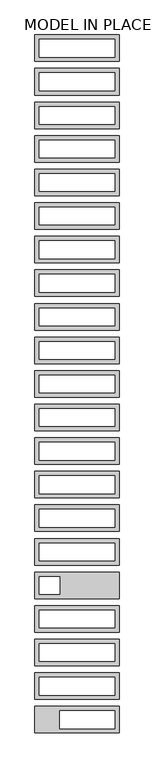
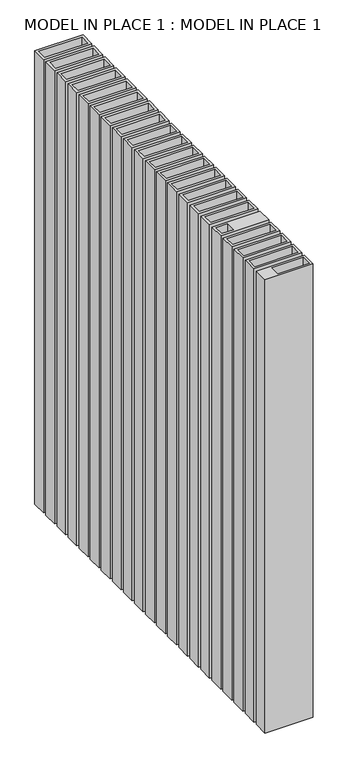
"""IFC4 building model written with IfcOpenShell, lengths in millimetres: proxy geometry, MODEL IN PLACE 1 : MODEL IN PLACE 1."""

from ifc_helpers import new_model, si_unit, frame, origin, place, context, project, spatial, polyline, outline, extrude, source, transform, mapped, element, save


def model_in_place_1_model_in_place_1_9ea038c9(model_context):
    return source(origin(), model_context, "Body", "SweptSolid", [
        extrude(outline(polyline([(-3736.8593778, -7719.7746485), (-3736.8593778, -7940.4371485), (-4436.9468778, -7940.4371485), (-4436.9468778, -7719.7746485), (-3736.8593778, -7719.7746485)]), holes=[polyline([(-3772.7765653, -7757.279336), (-4229.8015106, -7757.279336), (-4229.8015106, -7904.519961), (-3772.7765653, -7904.519961), (-3772.7765653, -7757.279336)])]), frame((0.0, 0.0, 35.9758221), z_axis=(0.0, 0.0, 1.0), x_axis=(1.0, 0.0, 0.0)), (0.0, 0.0, 1.0), 6974.2445714),
        extrude(outline(polyline([(-3736.8593778, -7440.3746485), (-3736.8593778, -7661.0371485), (-4436.9468778, -7661.0371485), (-4436.9468778, -7440.3746485), (-3736.8593778, -7440.3746485)]), holes=[polyline([(-3772.7765653, -7477.879336), (-4400.2359403, -7477.879336), (-4400.2359403, -7625.119961), (-3772.7765653, -7625.119961), (-3772.7765653, -7477.879336)])]), frame((0.0, 0.0, 35.9758221), z_axis=(0.0, 0.0, 1.0), x_axis=(1.0, 0.0, 0.0)), (0.0, 0.0, 1.0), 6974.2445714),
        extrude(outline(polyline([(-3736.8593778, -7160.9746485), (-3736.8593778, -7381.6371485), (-4436.9468778, -7381.6371485), (-4436.9468778, -7160.9746485), (-3736.8593778, -7160.9746485)]), holes=[polyline([(-3772.7765653, -7198.479336), (-4400.2359403, -7198.479336), (-4400.2359403, -7345.719961), (-3772.7765653, -7345.719961), (-3772.7765653, -7198.479336)])]), frame((0.0, 0.0, 35.9758221), z_axis=(0.0, 0.0, 1.0), x_axis=(1.0, 0.0, 0.0)), (0.0, 0.0, 1.0), 6974.2445714),
        extrude(outline(polyline([(-3736.8593778, -6881.5746485), (-3736.8593778, -7102.2371485), (-4436.9468778, -7102.2371485), (-4436.9468778, -6881.5746485), (-3736.8593778, -6881.5746485)]), holes=[polyline([(-3772.7765653, -6919.079336), (-4400.2359403, -6919.079336), (-4400.2359403, -7066.319961), (-3772.7765653, -7066.319961), (-3772.7765653, -6919.079336)])]), frame((0.0, 0.0, 35.9758221), z_axis=(0.0, 0.0, 1.0), x_axis=(1.0, 0.0, 0.0)), (0.0, 0.0, 1.0), 6974.2445714),
        extrude(outline(polyline([(-3736.8593778, -6602.1746485), (-3736.8593778, -6822.8371485), (-4436.9468778, -6822.8371485), (-4436.9468778, -6602.1746485), (-3736.8593778, -6602.1746485)]), holes=[polyline([(-4229.8015106, -6639.679336), (-4400.2359403, -6639.679336), (-4400.2359403, -6786.919961), (-4229.8015106, -6786.919961), (-4229.8015106, -6639.679336)])]), frame((0.0, 0.0, 35.9758221), z_axis=(0.0, 0.0, 1.0), x_axis=(1.0, 0.0, 0.0)), (0.0, 0.0, 1.0), 6974.2445714),
        extrude(outline(polyline([(-3736.8593778, -6322.7746485), (-3736.8593778, -6543.4371485), (-4436.9468778, -6543.4371485), (-4436.9468778, -6322.7746485), (-3736.8593778, -6322.7746485)]), holes=[polyline([(-3772.7765653, -6360.279336), (-4400.2359403, -6360.279336), (-4400.2359403, -6507.519961), (-3772.7765653, -6507.519961), (-3772.7765653, -6360.279336)])]), frame((0.0, 0.0, 35.9758221), z_axis=(0.0, 0.0, 1.0), x_axis=(1.0, 0.0, 0.0)), (0.0, 0.0, 1.0), 6974.2445714),
        extrude(outline(polyline([(-3736.8593778, -6043.3746485), (-3736.8593778, -6264.0371485), (-4436.9468778, -6264.0371485), (-4436.9468778, -6043.3746485), (-3736.8593778, -6043.3746485)]), holes=[polyline([(-3772.7765653, -6080.879336), (-4400.2359403, -6080.879336), (-4400.2359403, -6228.119961), (-3772.7765653, -6228.119961), (-3772.7765653, -6080.879336)])]), frame((0.0, 0.0, 35.9758221), z_axis=(0.0, 0.0, 1.0), x_axis=(1.0, 0.0, 0.0)), (0.0, 0.0, 1.0), 6974.2445714),
        extrude(outline(polyline([(-3736.8593778, -5763.9746485), (-3736.8593778, -5984.6371485), (-4436.9468778, -5984.6371485), (-4436.9468778, -5763.9746485), (-3736.8593778, -5763.9746485)]), holes=[polyline([(-3772.7765653, -5801.479336), (-4400.2359403, -5801.479336), (-4400.2359403, -5948.719961), (-3772.7765653, -5948.719961), (-3772.7765653, -5801.479336)])]), frame((0.0, 0.0, 35.9758221), z_axis=(0.0, 0.0, 1.0), x_axis=(1.0, 0.0, 0.0)), (0.0, 0.0, 1.0), 6974.2445714),
        extrude(outline(polyline([(-3736.8593778, -5484.5746485), (-3736.8593778, -5705.2371485), (-4436.9468778, -5705.2371485), (-4436.9468778, -5484.5746485), (-3736.8593778, -5484.5746485)]), holes=[polyline([(-3772.7765653, -5522.079336), (-4400.2359403, -5522.079336), (-4400.2359403, -5669.319961), (-3772.7765653, -5669.319961), (-3772.7765653, -5522.079336)])]), frame((0.0, 0.0, 35.9758221), z_axis=(0.0, 0.0, 1.0), x_axis=(1.0, 0.0, 0.0)), (0.0, 0.0, 1.0), 6974.2445714),
        extrude(outline(polyline([(-3736.8593778, -5205.1746485), (-3736.8593778, -5425.8371485), (-4436.9468778, -5425.8371485), (-4436.9468778, -5205.1746485), (-3736.8593778, -5205.1746485)]), holes=[polyline([(-3772.7765653, -5242.679336), (-4400.2359403, -5242.679336), (-4400.2359403, -5389.919961), (-3772.7765653, -5389.919961), (-3772.7765653, -5242.679336)])]), frame((0.0, 0.0, 35.9758221), z_axis=(0.0, 0.0, 1.0), x_axis=(1.0, 0.0, 0.0)), (0.0, 0.0, 1.0), 6974.2445714),
        extrude(outline(polyline([(-3736.8593778, -4925.7746485), (-3736.8593778, -5146.4371485), (-4436.9468778, -5146.4371485), (-4436.9468778, -4925.7746485), (-3736.8593778, -4925.7746485)]), holes=[polyline([(-3772.7765653, -4963.279336), (-4400.2359403, -4963.279336), (-4400.2359403, -5110.519961), (-3772.7765653, -5110.519961), (-3772.7765653, -4963.279336)])]), frame((0.0, 0.0, 35.9758221), z_axis=(0.0, 0.0, 1.0), x_axis=(1.0, 0.0, 0.0)), (0.0, 0.0, 1.0), 6974.2445714),
        extrude(outline(polyline([(-3736.8593778, -4646.3746485), (-3736.8593778, -4867.0371485), (-4436.9468778, -4867.0371485), (-4436.9468778, -4646.3746485), (-3736.8593778, -4646.3746485)]), holes=[polyline([(-3772.7765653, -4683.879336), (-4400.2359403, -4683.879336), (-4400.2359403, -4831.119961), (-3772.7765653, -4831.119961), (-3772.7765653, -4683.879336)])]), frame((0.0, 0.0, 35.9758221), z_axis=(0.0, 0.0, 1.0), x_axis=(1.0, 0.0, 0.0)), (0.0, 0.0, 1.0), 6974.2445714),
        extrude(outline(polyline([(-3736.8593778, -4366.9746485), (-3736.8593778, -4587.6371485), (-4436.9468778, -4587.6371485), (-4436.9468778, -4366.9746485), (-3736.8593778, -4366.9746485)]), holes=[polyline([(-3772.7765653, -4404.479336), (-4400.2359403, -4404.479336), (-4400.2359403, -4551.719961), (-3772.7765653, -4551.719961), (-3772.7765653, -4404.479336)])]), frame((0.0, 0.0, 35.9758221), z_axis=(0.0, 0.0, 1.0), x_axis=(1.0, 0.0, 0.0)), (0.0, 0.0, 1.0), 6974.2445714),
        extrude(outline(polyline([(-3736.8593778, -4087.5746485), (-3736.8593778, -4308.2371485), (-4436.9468778, -4308.2371485), (-4436.9468778, -4087.5746485), (-3736.8593778, -4087.5746485)]), holes=[polyline([(-3772.7765653, -4125.079336), (-4400.2359403, -4125.079336), (-4400.2359403, -4272.319961), (-3772.7765653, -4272.319961), (-3772.7765653, -4125.079336)])]), frame((0.0, 0.0, 35.9758221), z_axis=(0.0, 0.0, 1.0), x_axis=(1.0, 0.0, 0.0)), (0.0, 0.0, 1.0), 6974.2445714),
        extrude(outline(polyline([(-3736.8593778, -3808.1746485), (-3736.8593778, -4028.8371485), (-4436.9468778, -4028.8371485), (-4436.9468778, -3808.1746485), (-3736.8593778, -3808.1746485)]), holes=[polyline([(-3772.7765653, -3845.679336), (-4400.2359403, -3845.679336), (-4400.2359403, -3992.919961), (-3772.7765653, -3992.919961), (-3772.7765653, -3845.679336)])]), frame((0.0, 0.0, 35.9758221), z_axis=(0.0, 0.0, 1.0), x_axis=(1.0, 0.0, 0.0)), (0.0, 0.0, 1.0), 6974.2445714),
        extrude(outline(polyline([(-3736.8593778, -3528.7746485), (-3736.8593778, -3749.4371485), (-4436.9468778, -3749.4371485), (-4436.9468778, -3528.7746485), (-3736.8593778, -3528.7746485)]), holes=[polyline([(-3772.7765653, -3566.279336), (-4400.2359403, -3566.279336), (-4400.2359403, -3713.519961), (-3772.7765653, -3713.519961), (-3772.7765653, -3566.279336)])]), frame((0.0, 0.0, 35.9758221), z_axis=(0.0, 0.0, 1.0), x_axis=(1.0, 0.0, 0.0)), (0.0, 0.0, 1.0), 6974.2445714),
        extrude(outline(polyline([(-3736.8593778, -3249.3746485), (-3736.8593778, -3470.0371485), (-4436.9468778, -3470.0371485), (-4436.9468778, -3249.3746485), (-3736.8593778, -3249.3746485)]), holes=[polyline([(-3772.7765653, -3286.879336), (-4400.2359403, -3286.879336), (-4400.2359403, -3434.119961), (-3772.7765653, -3434.119961), (-3772.7765653, -3286.879336)])]), frame((0.0, 0.0, 35.9758221), z_axis=(0.0, 0.0, 1.0), x_axis=(1.0, 0.0, 0.0)), (0.0, 0.0, 1.0), 6974.2445714),
        extrude(outline(polyline([(-3736.8593778, -2969.9746485), (-3736.8593778, -3190.6371485), (-4436.9468778, -3190.6371485), (-4436.9468778, -2969.9746485), (-3736.8593778, -2969.9746485)]), holes=[polyline([(-3772.7765653, -3007.479336), (-4400.2359403, -3007.479336), (-4400.2359403, -3154.719961), (-3772.7765653, -3154.719961), (-3772.7765653, -3007.479336)])]), frame((0.0, 0.0, 35.9758221), z_axis=(0.0, 0.0, 1.0), x_axis=(1.0, 0.0, 0.0)), (0.0, 0.0, 1.0), 6974.2445714),
        extrude(outline(polyline([(-3736.8593778, -2690.5746485), (-3736.8593778, -2911.2371485), (-4436.9468778, -2911.2371485), (-4436.9468778, -2690.5746485), (-3736.8593778, -2690.5746485)]), holes=[polyline([(-3772.7765653, -2728.079336), (-4400.2359403, -2728.079336), (-4400.2359403, -2875.319961), (-3772.7765653, -2875.319961), (-3772.7765653, -2728.079336)])]), frame((0.0, 0.0, 35.9758221), z_axis=(0.0, 0.0, 1.0), x_axis=(1.0, 0.0, 0.0)), (0.0, 0.0, 1.0), 6974.2445714),
        extrude(outline(polyline([(-3736.8593778, -2411.1746485), (-3736.8593778, -2631.8371485), (-4436.9468778, -2631.8371485), (-4436.9468778, -2411.1746485), (-3736.8593778, -2411.1746485)]), holes=[polyline([(-3772.7765653, -2448.679336), (-4400.2359403, -2448.679336), (-4400.2359403, -2595.919961), (-3772.7765653, -2595.919961), (-3772.7765653, -2448.679336)])]), frame((0.0, 0.0, 35.9758221), z_axis=(0.0, 0.0, 1.0), x_axis=(1.0, 0.0, 0.0)), (0.0, 0.0, 1.0), 6974.2445714),
        extrude(outline(polyline([(-3736.8593778, -2131.7746485), (-3736.8593778, -2352.4371485), (-4436.9468778, -2352.4371485), (-4436.9468778, -2131.7746485), (-3736.8593778, -2131.7746485)]), holes=[polyline([(-3772.7765653, -2169.279336), (-4400.2359403, -2169.279336), (-4400.2359403, -2316.519961), (-3772.7765653, -2316.519961), (-3772.7765653, -2169.279336)])]), frame((0.0, 0.0, 35.9758221), z_axis=(0.0, 0.0, 1.0), x_axis=(1.0, 0.0, 0.0)), (0.0, 0.0, 1.0), 6974.2445714),
    ])


if __name__ == "__main__":
    model = new_model("IFC4")
    model_context = context("Model", 3, world=origin())
    ifc_project = project(units=[si_unit("LENGTHUNIT", "METRE", prefix="MILLI")], contexts=[model_context])
    site = spatial("IfcSite", under=ifc_project)
    building = spatial("IfcBuilding", under=site)
    placement = place(None, origin())
    model_in_place_1_model_in_place_1_shape = model_in_place_1_model_in_place_1_9ea038c9(model_context)
    element("IfcBuildingElementProxy", 1, Name="MODEL IN PLACE 1 : MODEL IN PLACE 1", ObjectType="MODEL IN PLACE 1 : MODEL IN PLACE 1", at=placement, inside=building, context=model_context, shape_type="MappedRepresentation", body=[
        mapped(model_in_place_1_model_in_place_1_shape, transform((0.0, 0.0, 0.0), x_axis=(1.0, 0.0, 0.0), y_axis=(0.0, 1.0, 0.0), z_axis=(0.0, 0.0, 1.0))),
    ])
    save(model, "model.ifc")
